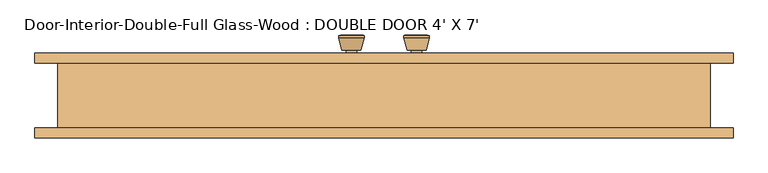
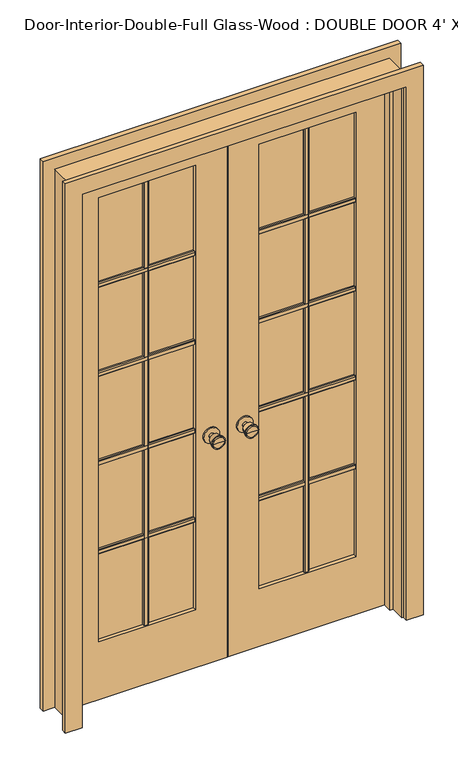
"""IFC4 building model written with IfcOpenShell, lengths in millimetres: door geometry, Door-Interior-Double-Full Glass-Wood : DOUBLE DOOR 4' X 7'."""

from ifc_helpers import new_model, si_unit, point, frame, frame_2d, origin, place, context, project, spatial, polyline, circle_curve, trimmed, segment, composite_curve, outline, extrude, faceted_brep, source, transform, mapped, element, save
from ifc_brep_helpers import plane_surface, cylinder_surface, revolved_surface, advanced_brep


def door_interior_double_full_glass_wood_double_door_4_x_7_060eee9d(model_context):
    return source(origin(), model_context, "Body", "SolidModel", [
        advanced_brep(
        [(-63.5, 66.325, 914.4), (-73.5, 66.325, 914.4), (-53.5, 66.325, 914.4), (-83.9758676, 115.325, 914.4), (-63.5, 115.325, 914.4), (-43.0241324, 115.325, 914.4), (-88.5, 113.4971319, 914.4), (-38.5, 113.4971319, 914.4), (-88.5, 110.0334537, 914.4), (-38.5, 110.0334537, 914.4), (-82.136236, 85.325, 914.4), (-44.863764, 85.325, 914.4), (-73.5, 85.325, 914.4), (-53.5, 85.325, 914.4)],
        [
            (0, 1),
            (1, 2, circle_curve(frame((-63.5, 66.325, 914.4), z_axis=(0.0, -1.0, 0.0), x_axis=(1.0, 0.0, 0.0)), 10.0)),
            (2, 0),
            (2, 1, circle_curve(frame((-63.5, 66.325, 914.4), z_axis=(0.0, -1.0, 0.0), x_axis=(1.0, 0.0, 0.0)), 10.0)),
            (3, 4),
            (4, 5),
            (5, 3, circle_curve(frame((-63.5, 115.325, 914.4), z_axis=(0.0, 1.0, 0.0), x_axis=(1.0, 0.0, 0.0)), 20.4758676)),
            (3, 5, circle_curve(frame((-63.5, 115.325, 914.4), z_axis=(0.0, 1.0, 0.0), x_axis=(1.0, 0.0, 0.0)), 20.4758676)),
            (6, 3),
            (5, 7),
            (7, 6, circle_curve(frame((-63.5, 113.4971319, 914.4), z_axis=(0.0, 1.0, 0.0), x_axis=(1.0, 0.0, 0.0)), 25.0)),
            (6, 7, circle_curve(frame((-63.5, 113.4971319, 914.4), z_axis=(0.0, 1.0, 0.0), x_axis=(1.0, 0.0, 0.0)), 25.0)),
            (8, 6),
            (7, 9),
            (9, 8, circle_curve(frame((-63.5, 110.0334537, 914.4), z_axis=(0.0, 1.0, 0.0), x_axis=(1.0, 0.0, 0.0)), 25.0)),
            (8, 9, circle_curve(frame((-63.5, 110.0334537, 914.4), z_axis=(0.0, 1.0, 0.0), x_axis=(1.0, 0.0, 0.0)), 25.0)),
            (10, 8),
            (9, 11),
            (11, 10, circle_curve(frame((-63.5, 85.325, 914.4), z_axis=(0.0, 1.0, 0.0), x_axis=(1.0, 0.0, 0.0)), 18.636236)),
            (10, 11, circle_curve(frame((-63.5, 85.325, 914.4), z_axis=(0.0, 1.0, 0.0), x_axis=(1.0, 0.0, 0.0)), 18.636236)),
            (12, 10),
            (11, 13),
            (13, 12, circle_curve(frame((-63.5, 85.325, 914.4), z_axis=(0.0, 1.0, 0.0), x_axis=(1.0, 0.0, 0.0)), 10.0)),
            (12, 13, circle_curve(frame((-63.5, 85.325, 914.4), z_axis=(0.0, 1.0, 0.0), x_axis=(1.0, 0.0, 0.0)), 10.0)),
            (1, 12),
            (13, 2),
        ],
        [
            plane_surface(frame((-63.5, 66.325, 914.4), z_axis=(0.0, -1.0, 0.0), x_axis=(1.0, 0.0, 0.0))),
            plane_surface(frame((-63.5, 115.325, 914.4), z_axis=(0.0, 1.0, 0.0), x_axis=(1.0, 0.0, 0.0))),
            revolved_surface(polyline([(-43.0241324, 115.325, 914.4), (-38.5, 113.4971319, 914.4)]), (-63.5, 66.325, 914.4), (0.0, -1.0, 0.0)),
            cylinder_surface(frame((-63.5, 66.325, 914.4), z_axis=(0.0, -1.0, 0.0), x_axis=(1.0, 0.0, 0.0)), 25.0),
            revolved_surface(polyline([(-38.5, 110.0334537, 914.4), (-44.863764, 85.325, 914.4)]), (-63.5, 66.325, 914.4), (0.0, -1.0, 0.0)),
            plane_surface(frame((-63.5, 85.325, 914.4), z_axis=(0.0, -1.0, 0.0), x_axis=(1.0, 0.0, 0.0))),
            cylinder_surface(frame((-63.5, 66.325, 914.4), z_axis=(0.0, -1.0, 0.0), x_axis=(1.0, 0.0, 0.0)), 10.0),
        ],
        [
            (0, [[1, 2, 3]]),
            (0, [[-3, 4, -1]]),
            (1, [[5, 6, 7]]),
            (1, [[-6, -5, 8]]),
            (2, [[9, -7, 10, 11]]),
            (2, [[-10, -8, -9, 12]]),
            (3, [[13, -11, 14, 15]]),
            (3, [[-14, -12, -13, 16]]),
            (4, [[17, -15, 18, 19]]),
            (4, [[-18, -16, -17, 20]]),
            (5, [[21, -19, 22, 23]]),
            (5, [[-22, -20, -21, 24]]),
            (6, [[25, -23, 26, -2]]),
            (6, [[-26, -24, -25, -4]]),
        ],
    ),
        extrude(outline(composite_curve([segment(trimmed(circle_curve(frame_2d((914.4, -63.5)), 30.0), [point((914.4, -33.5))], [point((914.4, -93.5))], False, "CARTESIAN"), True, "CONTINUOUS"), segment(trimmed(circle_curve(frame_2d((914.4, -63.5)), 30.0), [point((914.4, -93.5))], [point((914.4, -33.5))], False, "CARTESIAN"), True, "CONTINUOUS")], self_intersect=False)), frame((0.0, 60.325, 0.0), z_axis=(0.0, 1.0, 0.0), x_axis=(0.0, 0.0, 1.0)), (0.0, 0.0, 1.0), 6.0),
        advanced_brep(
        [(-63.5, 19.4, 914.4), (-53.5, 19.4, 914.4), (-73.5, 19.4, 914.4), (-83.9758676, -29.6, 914.4), (-43.0241324, -29.6, 914.4), (-63.5, -29.6, 914.4), (-88.5, -27.7721319, 914.4), (-38.5, -27.7721319, 914.4), (-88.5, -24.3084537, 914.4), (-38.5, -24.3084537, 914.4), (-82.136236, 0.4, 914.4), (-44.863764, 0.4, 914.4), (-73.5, 0.4, 914.4), (-53.5, 0.4, 914.4)],
        [
            (0, 1),
            (1, 2, circle_curve(frame((-63.5, 19.4, 914.4), z_axis=(0.0, 1.0, 0.0), x_axis=(1.0, 0.0, 0.0)), 10.0)),
            (2, 0),
            (2, 1, circle_curve(frame((-63.5, 19.4, 914.4), z_axis=(0.0, 1.0, 0.0), x_axis=(1.0, 0.0, 0.0)), 10.0)),
            (3, 4, circle_curve(frame((-63.5, -29.6, 914.4), z_axis=(0.0, -1.0, 0.0), x_axis=(1.0, 0.0, 0.0)), 20.4758676)),
            (4, 5),
            (5, 3),
            (4, 3, circle_curve(frame((-63.5, -29.6, 914.4), z_axis=(0.0, -1.0, 0.0), x_axis=(1.0, 0.0, 0.0)), 20.4758676)),
            (6, 7, circle_curve(frame((-63.5, -27.7721319, 914.4), z_axis=(0.0, -1.0, 0.0), x_axis=(1.0, 0.0, 0.0)), 25.0)),
            (7, 4),
            (3, 6),
            (7, 6, circle_curve(frame((-63.5, -27.7721319, 914.4), z_axis=(0.0, -1.0, 0.0), x_axis=(1.0, 0.0, 0.0)), 25.0)),
            (8, 9, circle_curve(frame((-63.5, -24.3084537, 914.4), z_axis=(0.0, -1.0, 0.0), x_axis=(1.0, 0.0, 0.0)), 25.0)),
            (9, 7),
            (6, 8),
            (9, 8, circle_curve(frame((-63.5, -24.3084537, 914.4), z_axis=(0.0, -1.0, 0.0), x_axis=(1.0, 0.0, 0.0)), 25.0)),
            (10, 11, circle_curve(frame((-63.5, 0.4, 914.4), z_axis=(0.0, -1.0, 0.0), x_axis=(1.0, 0.0, 0.0)), 18.636236)),
            (11, 9),
            (8, 10),
            (11, 10, circle_curve(frame((-63.5, 0.4, 914.4), z_axis=(0.0, -1.0, 0.0), x_axis=(1.0, 0.0, 0.0)), 18.636236)),
            (12, 13, circle_curve(frame((-63.5, 0.4, 914.4), z_axis=(0.0, -1.0, 0.0), x_axis=(1.0, 0.0, 0.0)), 10.0)),
            (13, 11),
            (10, 12),
            (13, 12, circle_curve(frame((-63.5, 0.4, 914.4), z_axis=(0.0, -1.0, 0.0), x_axis=(1.0, 0.0, 0.0)), 10.0)),
            (1, 13),
            (12, 2),
        ],
        [
            plane_surface(frame((-63.5, 19.4, 914.4), z_axis=(0.0, 1.0, 0.0), x_axis=(1.0, 0.0, 0.0))),
            plane_surface(frame((-63.5, -29.6, 914.4), z_axis=(0.0, -1.0, 0.0), x_axis=(1.0, 0.0, 0.0))),
            revolved_surface(polyline([(-43.0241324, -29.6, 914.4), (-38.5, -27.7721319, 914.4)]), (-63.5, 19.4, 914.4), (0.0, 1.0, 0.0)),
            cylinder_surface(frame((-63.5, 19.4, 914.4), z_axis=(0.0, 1.0, 0.0), x_axis=(1.0, 0.0, 0.0)), 25.0),
            revolved_surface(polyline([(-38.5, -24.3084537, 914.4), (-44.863764, 0.4, 914.4)]), (-63.5, 19.4, 914.4), (0.0, 1.0, 0.0)),
            plane_surface(frame((-63.5, 0.4, 914.4), z_axis=(0.0, 1.0, 0.0), x_axis=(1.0, 0.0, 0.0))),
            cylinder_surface(frame((-63.5, 19.4, 914.4), z_axis=(0.0, 1.0, 0.0), x_axis=(1.0, 0.0, 0.0)), 10.0),
        ],
        [
            (0, [[1, 2, 3]]),
            (0, [[-3, 4, -1]]),
            (1, [[5, 6, 7]]),
            (1, [[8, -7, -6]]),
            (2, [[9, 10, -5, 11]]),
            (2, [[12, -11, -8, -10]]),
            (3, [[13, 14, -9, 15]]),
            (3, [[16, -15, -12, -14]]),
            (4, [[17, 18, -13, 19]]),
            (4, [[20, -19, -16, -18]]),
            (5, [[21, 22, -17, 23]]),
            (5, [[24, -23, -20, -22]]),
            (6, [[-2, 25, -21, 26]]),
            (6, [[-4, -26, -24, -25]]),
        ],
    ),
        extrude(outline(composite_curve([segment(trimmed(circle_curve(frame_2d((914.4, -63.5)), 30.0), [point((914.4, -33.5))], [point((914.4, -93.5))], False, "CARTESIAN"), True, "CONTINUOUS"), segment(trimmed(circle_curve(frame_2d((914.4, -63.5)), 30.0), [point((914.4, -93.5))], [point((914.4, -33.5))], False, "CARTESIAN"), True, "CONTINUOUS")], self_intersect=False)), frame((0.0, 19.4, 0.0), z_axis=(0.0, 1.0, 0.0), x_axis=(0.0, 0.0, 1.0)), (0.0, 0.0, 1.0), 6.0),
        extrude(outline(polyline([(39.37, 1667.51), (39.37, 1648.46), (33.02, 1648.46), (29.845, 1651.635), (29.845, 1664.335), (33.02, 1667.51), (39.37, 1667.51)])), frame((120.65, 0.0, 0.0), z_axis=(1.0, 0.0, 0.0), x_axis=(0.0, 1.0, 0.0)), (0.0, 0.0, 1.0), 368.3),
        extrude(outline(polyline([(39.37, 1310.9575), (39.37, 1291.9075), (33.02, 1291.9075), (29.845, 1295.0825), (29.845, 1307.7825), (33.02, 1310.9575), (39.37, 1310.9575)])), frame((120.65, 0.0, 0.0), z_axis=(1.0, 0.0, 0.0), x_axis=(0.0, 1.0, 0.0)), (0.0, 0.0, 1.0), 368.3),
        extrude(outline(polyline([(39.37, 954.405), (39.37, 935.355), (33.02, 935.355), (29.845, 938.53), (29.845, 951.23), (33.02, 954.405), (39.37, 954.405)])), frame((120.65, 0.0, 0.0), z_axis=(1.0, 0.0, 0.0), x_axis=(0.0, 1.0, 0.0)), (0.0, 0.0, 1.0), 368.3),
        extrude(outline(polyline([(295.275, 39.37), (314.325, 39.37), (314.325, 33.02), (311.15, 29.845), (298.45, 29.845), (295.275, 33.02), (295.275, 39.37)])), frame((0.0, 0.0, 231.775), z_axis=(0.0, 0.0, 1.0), x_axis=(1.0, 0.0, 0.0)), (0.0, 0.0, 1.0), 1782.7625),
        extrude(outline(polyline([(39.37, 597.8525), (39.37, 578.8025), (33.02, 578.8025), (29.845, 581.9775), (29.845, 594.6775), (33.02, 597.8525), (39.37, 597.8525)])), frame((120.65, 0.0, 0.0), z_axis=(1.0, 0.0, 0.0), x_axis=(0.0, 1.0, 0.0)), (0.0, 0.0, 1.0), 368.3),
        extrude(outline(polyline([(46.355, 1667.51), (52.705, 1667.51), (55.88, 1664.335), (55.88, 1651.635), (52.705, 1648.46), (46.355, 1648.46), (46.355, 1667.51)])), frame((-488.95, 0.0, 0.0), z_axis=(1.0, 0.0, 0.0), x_axis=(0.0, 1.0, 0.0)), (0.0, 0.0, 1.0), 368.3),
        extrude(outline(polyline([(46.355, 1310.9575), (52.705, 1310.9575), (55.88, 1307.7825), (55.88, 1295.0825), (52.705, 1291.9075), (46.355, 1291.9075), (46.355, 1310.9575)])), frame((-488.95, 0.0, 0.0), z_axis=(1.0, 0.0, 0.0), x_axis=(0.0, 1.0, 0.0)), (0.0, 0.0, 1.0), 368.3),
        extrude(outline(polyline([(46.355, 954.405), (52.705, 954.405), (55.88, 951.23), (55.88, 938.53), (52.705, 935.355), (46.355, 935.355), (46.355, 954.405)])), frame((-488.95, 0.0, 0.0), z_axis=(1.0, 0.0, 0.0), x_axis=(0.0, 1.0, 0.0)), (0.0, 0.0, 1.0), 368.3),
        extrude(outline(polyline([(-314.325, 46.355), (-314.325, 52.705), (-311.15, 55.88), (-298.45, 55.88), (-295.275, 52.705), (-295.275, 46.355), (-314.325, 46.355)])), frame((0.0, 0.0, 231.775), z_axis=(0.0, 0.0, 1.0), x_axis=(1.0, 0.0, 0.0)), (0.0, 0.0, 1.0), 1782.7625),
        extrude(outline(polyline([(46.355, 597.8525), (52.705, 597.8525), (55.88, 594.6775), (55.88, 581.9775), (52.705, 578.8025), (46.355, 578.8025), (46.355, 597.8525)])), frame((-488.95, 0.0, 0.0), z_axis=(1.0, 0.0, 0.0), x_axis=(0.0, 1.0, 0.0)), (0.0, 0.0, 1.0), 368.3),
        extrude(outline(polyline([(46.355, 1667.51), (52.705, 1667.51), (55.88, 1664.335), (55.88, 1651.635), (52.705, 1648.46), (46.355, 1648.46), (46.355, 1667.51)])), frame((120.65, 0.0, 0.0), z_axis=(1.0, 0.0, 0.0), x_axis=(0.0, 1.0, 0.0)), (0.0, 0.0, 1.0), 368.3),
        extrude(outline(polyline([(46.355, 1310.9575), (52.705, 1310.9575), (55.88, 1307.7825), (55.88, 1295.0825), (52.705, 1291.9075), (46.355, 1291.9075), (46.355, 1310.9575)])), frame((120.65, 0.0, 0.0), z_axis=(1.0, 0.0, 0.0), x_axis=(0.0, 1.0, 0.0)), (0.0, 0.0, 1.0), 368.3),
        extrude(outline(polyline([(46.355, 954.405), (52.705, 954.405), (55.88, 951.23), (55.88, 938.53), (52.705, 935.355), (46.355, 935.355), (46.355, 954.405)])), frame((120.65, 0.0, 0.0), z_axis=(1.0, 0.0, 0.0), x_axis=(0.0, 1.0, 0.0)), (0.0, 0.0, 1.0), 368.3),
        extrude(outline(polyline([(295.275, 46.355), (295.275, 52.705), (298.45, 55.88), (311.15, 55.88), (314.325, 52.705), (314.325, 46.355), (295.275, 46.355)])), frame((0.0, 0.0, 231.775), z_axis=(0.0, 0.0, 1.0), x_axis=(1.0, 0.0, 0.0)), (0.0, 0.0, 1.0), 1782.7625),
        extrude(outline(polyline([(46.355, 597.8525), (52.705, 597.8525), (55.88, 594.6775), (55.88, 581.9775), (52.705, 578.8025), (46.355, 578.8025), (46.355, 597.8525)])), frame((120.65, 0.0, 0.0), z_axis=(1.0, 0.0, 0.0), x_axis=(0.0, 1.0, 0.0)), (0.0, 0.0, 1.0), 368.3),
        extrude(outline(polyline([(39.37, 1667.51), (39.37, 1648.46), (33.02, 1648.46), (29.845, 1651.635), (29.845, 1664.335), (33.02, 1667.51), (39.37, 1667.51)])), frame((-488.95, 0.0, 0.0), z_axis=(1.0, 0.0, 0.0), x_axis=(0.0, 1.0, 0.0)), (0.0, 0.0, 1.0), 368.3),
        extrude(outline(polyline([(39.37, 1310.9575), (39.37, 1291.9075), (33.02, 1291.9075), (29.845, 1295.0825), (29.845, 1307.7825), (33.02, 1310.9575), (39.37, 1310.9575)])), frame((-488.95, 0.0, 0.0), z_axis=(1.0, 0.0, 0.0), x_axis=(0.0, 1.0, 0.0)), (0.0, 0.0, 1.0), 368.3),
        extrude(outline(polyline([(39.37, 954.405), (39.37, 935.355), (33.02, 935.355), (29.845, 938.53), (29.845, 951.23), (33.02, 954.405), (39.37, 954.405)])), frame((-488.95, 0.0, 0.0), z_axis=(1.0, 0.0, 0.0), x_axis=(0.0, 1.0, 0.0)), (0.0, 0.0, 1.0), 368.3),
        extrude(outline(polyline([(-314.325, 39.37), (-295.275, 39.37), (-295.275, 33.02), (-298.45, 29.845), (-311.15, 29.845), (-314.325, 33.02), (-314.325, 39.37)])), frame((0.0, 0.0, 231.775), z_axis=(0.0, 0.0, 1.0), x_axis=(1.0, 0.0, 0.0)), (0.0, 0.0, 1.0), 1782.7625),
        extrude(outline(polyline([(39.37, 597.8525), (39.37, 578.8025), (33.02, 578.8025), (29.845, 581.9775), (29.845, 594.6775), (33.02, 597.8525), (39.37, 597.8525)])), frame((-488.95, 0.0, 0.0), z_axis=(1.0, 0.0, 0.0), x_axis=(0.0, 1.0, 0.0)), (0.0, 0.0, 1.0), 368.3),
        advanced_brep(
        [(63.5, 19.4, 914.4), (73.5, 19.4, 914.4), (53.5, 19.4, 914.4), (83.9758676, -29.6, 914.4), (63.5, -29.6, 914.4), (43.0241324, -29.6, 914.4), (88.5, -27.7721319, 914.4), (38.5, -27.7721319, 914.4), (88.5, -24.3084537, 914.4), (38.5, -24.3084537, 914.4), (82.136236, 0.4, 914.4), (44.863764, 0.4, 914.4), (73.5, 0.4, 914.4), (53.5, 0.4, 914.4)],
        [
            (0, 1),
            (1, 2, circle_curve(frame((63.5, 19.4, 914.4), z_axis=(0.0, 1.0, 0.0), x_axis=(-1.0, 0.0, 0.0)), 10.0)),
            (2, 0),
            (2, 1, circle_curve(frame((63.5, 19.4, 914.4), z_axis=(0.0, 1.0, 0.0), x_axis=(-1.0, 0.0, 0.0)), 10.0)),
            (3, 4),
            (4, 5),
            (5, 3, circle_curve(frame((63.5, -29.6, 914.4), z_axis=(0.0, -1.0, 0.0), x_axis=(-1.0, 0.0, 0.0)), 20.4758676)),
            (3, 5, circle_curve(frame((63.5, -29.6, 914.4), z_axis=(0.0, -1.0, 0.0), x_axis=(-1.0, 0.0, 0.0)), 20.4758676)),
            (6, 3),
            (5, 7),
            (7, 6, circle_curve(frame((63.5, -27.7721319, 914.4), z_axis=(0.0, -1.0, 0.0), x_axis=(-1.0, 0.0, 0.0)), 25.0)),
            (6, 7, circle_curve(frame((63.5, -27.7721319, 914.4), z_axis=(0.0, -1.0, 0.0), x_axis=(-1.0, 0.0, 0.0)), 25.0)),
            (8, 6),
            (7, 9),
            (9, 8, circle_curve(frame((63.5, -24.3084537, 914.4), z_axis=(0.0, -1.0, 0.0), x_axis=(-1.0, 0.0, 0.0)), 25.0)),
            (8, 9, circle_curve(frame((63.5, -24.3084537, 914.4), z_axis=(0.0, -1.0, 0.0), x_axis=(-1.0, 0.0, 0.0)), 25.0)),
            (10, 8),
            (9, 11),
            (11, 10, circle_curve(frame((63.5, 0.4, 914.4), z_axis=(0.0, -1.0, 0.0), x_axis=(-1.0, 0.0, 0.0)), 18.636236)),
            (10, 11, circle_curve(frame((63.5, 0.4, 914.4), z_axis=(0.0, -1.0, 0.0), x_axis=(-1.0, 0.0, 0.0)), 18.636236)),
            (12, 10),
            (11, 13),
            (13, 12, circle_curve(frame((63.5, 0.4, 914.4), z_axis=(0.0, -1.0, 0.0), x_axis=(-1.0, 0.0, 0.0)), 10.0)),
            (12, 13, circle_curve(frame((63.5, 0.4, 914.4), z_axis=(0.0, -1.0, 0.0), x_axis=(-1.0, 0.0, 0.0)), 10.0)),
            (1, 12),
            (13, 2),
        ],
        [
            plane_surface(frame((63.5, 19.4, 914.4), z_axis=(0.0, 1.0, 0.0), x_axis=(-1.0, 0.0, 0.0))),
            plane_surface(frame((63.5, -29.6, 914.4), z_axis=(0.0, -1.0, 0.0), x_axis=(-1.0, 0.0, 0.0))),
            revolved_surface(polyline([(43.0241324, -29.6, 914.4), (38.5, -27.7721319, 914.4)]), (63.5, 19.4, 914.4), (0.0, 1.0, 0.0)),
            cylinder_surface(frame((63.5, 19.4, 914.4), z_axis=(0.0, 1.0, 0.0), x_axis=(-1.0, 0.0, 0.0)), 25.0),
            revolved_surface(polyline([(38.5, -24.3084537, 914.4), (44.863764, 0.4, 914.4)]), (63.5, 19.4, 914.4), (0.0, 1.0, 0.0)),
            plane_surface(frame((63.5, 0.4, 914.4), z_axis=(0.0, 1.0, 0.0), x_axis=(-1.0, 0.0, 0.0))),
            cylinder_surface(frame((63.5, 19.4, 914.4), z_axis=(0.0, 1.0, 0.0), x_axis=(-1.0, 0.0, 0.0)), 10.0),
        ],
        [
            (0, [[1, 2, 3]]),
            (0, [[-3, 4, -1]]),
            (1, [[5, 6, 7]]),
            (1, [[-6, -5, 8]]),
            (2, [[9, -7, 10, 11]]),
            (2, [[-10, -8, -9, 12]]),
            (3, [[13, -11, 14, 15]]),
            (3, [[-14, -12, -13, 16]]),
            (4, [[17, -15, 18, 19]]),
            (4, [[-18, -16, -17, 20]]),
            (5, [[21, -19, 22, 23]]),
            (5, [[-22, -20, -21, 24]]),
            (6, [[25, -23, 26, -2]]),
            (6, [[-26, -24, -25, -4]]),
        ],
    ),
        extrude(outline(composite_curve([segment(trimmed(circle_curve(frame_2d((914.4, 63.5)), 30.0), [point((914.4, 33.5))], [point((914.4, 93.5))], False, "CARTESIAN"), True, "CONTINUOUS"), segment(trimmed(circle_curve(frame_2d((914.4, 63.5)), 30.0), [point((914.4, 93.5))], [point((914.4, 33.5))], False, "CARTESIAN"), True, "CONTINUOUS")], self_intersect=False)), frame((0.0, 19.4, 0.0), z_axis=(0.0, 1.0, 0.0), x_axis=(0.0, 0.0, 1.0)), (0.0, 0.0, 1.0), 6.0),
        advanced_brep(
        [(63.5, 66.325, 914.4), (53.5, 66.325, 914.4), (73.5, 66.325, 914.4), (83.9758676, 115.325, 914.4), (43.0241324, 115.325, 914.4), (63.5, 115.325, 914.4), (88.5, 113.4971319, 914.4), (38.5, 113.4971319, 914.4), (88.5, 110.0334537, 914.4), (38.5, 110.0334537, 914.4), (82.136236, 85.325, 914.4), (44.863764, 85.325, 914.4), (73.5, 85.325, 914.4), (53.5, 85.325, 914.4)],
        [
            (0, 1),
            (1, 2, circle_curve(frame((63.5, 66.325, 914.4), z_axis=(0.0, -1.0, 0.0), x_axis=(-1.0, 0.0, 0.0)), 10.0)),
            (2, 0),
            (2, 1, circle_curve(frame((63.5, 66.325, 914.4), z_axis=(0.0, -1.0, 0.0), x_axis=(-1.0, 0.0, 0.0)), 10.0)),
            (3, 4, circle_curve(frame((63.5, 115.325, 914.4), z_axis=(0.0, 1.0, 0.0), x_axis=(-1.0, 0.0, 0.0)), 20.4758676)),
            (4, 5),
            (5, 3),
            (4, 3, circle_curve(frame((63.5, 115.325, 914.4), z_axis=(0.0, 1.0, 0.0), x_axis=(-1.0, 0.0, 0.0)), 20.4758676)),
            (6, 7, circle_curve(frame((63.5, 113.4971319, 914.4), z_axis=(0.0, 1.0, 0.0), x_axis=(-1.0, 0.0, 0.0)), 25.0)),
            (7, 4),
            (3, 6),
            (7, 6, circle_curve(frame((63.5, 113.4971319, 914.4), z_axis=(0.0, 1.0, 0.0), x_axis=(-1.0, 0.0, 0.0)), 25.0)),
            (8, 9, circle_curve(frame((63.5, 110.0334537, 914.4), z_axis=(0.0, 1.0, 0.0), x_axis=(-1.0, 0.0, 0.0)), 25.0)),
            (9, 7),
            (6, 8),
            (9, 8, circle_curve(frame((63.5, 110.0334537, 914.4), z_axis=(0.0, 1.0, 0.0), x_axis=(-1.0, 0.0, 0.0)), 25.0)),
            (10, 11, circle_curve(frame((63.5, 85.325, 914.4), z_axis=(0.0, 1.0, 0.0), x_axis=(-1.0, 0.0, 0.0)), 18.636236)),
            (11, 9),
            (8, 10),
            (11, 10, circle_curve(frame((63.5, 85.325, 914.4), z_axis=(0.0, 1.0, 0.0), x_axis=(-1.0, 0.0, 0.0)), 18.636236)),
            (12, 13, circle_curve(frame((63.5, 85.325, 914.4), z_axis=(0.0, 1.0, 0.0), x_axis=(-1.0, 0.0, 0.0)), 10.0)),
            (13, 11),
            (10, 12),
            (13, 12, circle_curve(frame((63.5, 85.325, 914.4), z_axis=(0.0, 1.0, 0.0), x_axis=(-1.0, 0.0, 0.0)), 10.0)),
            (1, 13),
            (12, 2),
        ],
        [
            plane_surface(frame((63.5, 66.325, 914.4), z_axis=(0.0, -1.0, 0.0), x_axis=(-1.0, 0.0, 0.0))),
            plane_surface(frame((63.5, 115.325, 914.4), z_axis=(0.0, 1.0, 0.0), x_axis=(-1.0, 0.0, 0.0))),
            revolved_surface(polyline([(43.0241324, 115.325, 914.4), (38.5, 113.4971319, 914.4)]), (63.5, 66.325, 914.4), (0.0, -1.0, 0.0)),
            cylinder_surface(frame((63.5, 66.325, 914.4), z_axis=(0.0, -1.0, 0.0), x_axis=(-1.0, 0.0, 0.0)), 25.0),
            revolved_surface(polyline([(38.5, 110.0334537, 914.4), (44.863764, 85.325, 914.4)]), (63.5, 66.325, 914.4), (0.0, -1.0, 0.0)),
            plane_surface(frame((63.5, 85.325, 914.4), z_axis=(0.0, -1.0, 0.0), x_axis=(-1.0, 0.0, 0.0))),
            cylinder_surface(frame((63.5, 66.325, 914.4), z_axis=(0.0, -1.0, 0.0), x_axis=(-1.0, 0.0, 0.0)), 10.0),
        ],
        [
            (0, [[1, 2, 3]]),
            (0, [[-3, 4, -1]]),
            (1, [[5, 6, 7]]),
            (1, [[8, -7, -6]]),
            (2, [[9, 10, -5, 11]]),
            (2, [[12, -11, -8, -10]]),
            (3, [[13, 14, -9, 15]]),
            (3, [[16, -15, -12, -14]]),
            (4, [[17, 18, -13, 19]]),
            (4, [[20, -19, -16, -18]]),
            (5, [[21, 22, -17, 23]]),
            (5, [[24, -23, -20, -22]]),
            (6, [[-2, 25, -21, 26]]),
            (6, [[-4, -26, -24, -25]]),
        ],
    ),
        extrude(outline(composite_curve([segment(trimmed(circle_curve(frame_2d((914.4, 63.5)), 30.0), [point((914.4, 33.5))], [point((914.4, 93.5))], False, "CARTESIAN"), True, "CONTINUOUS"), segment(trimmed(circle_curve(frame_2d((914.4, 63.5)), 30.0), [point((914.4, 93.5))], [point((914.4, 33.5))], False, "CARTESIAN"), True, "CONTINUOUS")], self_intersect=False)), frame((0.0, 60.325, 0.0), z_axis=(0.0, 1.0, 0.0), x_axis=(0.0, 0.0, 1.0)), (0.0, 0.0, 1.0), 6.0),
        extrude(outline(polyline([(0.0, 615.95), (0.0, 679.45), (2203.45, 679.45), (2203.45, -679.45), (0.0, -679.45), (0.0, -615.95), (2139.95, -615.95), (2139.95, 615.95), (0.0, 615.95)])), frame((0.0, -85.725, 0.0), z_axis=(0.0, 1.0, 0.0), x_axis=(0.0, 0.0, 1.0)), (0.0, 0.0, 1.0), 19.05),
        extrude(outline(polyline([(0.0, 615.95), (0.0, 679.45), (2203.45, 679.45), (2203.45, -679.45), (0.0, -679.45), (0.0, -615.95), (2139.95, -615.95), (2139.95, 615.95), (0.0, 615.95)])), frame((0.0, 60.325, 0.0), z_axis=(0.0, 1.0, 0.0), x_axis=(0.0, 0.0, 1.0)), (0.0, 0.0, 1.0), 19.05),
        faceted_brep([(635.0, 60.325, 0.0), (635.0, -66.675, 0.0), (609.6, -66.675, 0.0), (609.6, -9.525, 0.0), (596.9, -9.525, 0.0), (596.9, 25.4, 0.0), (609.6, 25.4, 0.0), (609.6, 60.325, 0.0), (635.0, 60.325, 2159.0), (635.0, -66.675, 2159.0), (-635.0, -66.675, 2159.0), (-635.0, -66.675, 0.0), (-609.6, -66.675, 0.0), (-609.6, -66.675, 2133.6), (609.6, -66.675, 2133.6), (609.6, -9.525, 2133.6), (-609.6, -9.525, 2133.6), (-609.6, -9.525, 0.0), (-596.9, -9.525, 0.0), (-596.9, -9.525, 2120.9), (596.9, -9.525, 2120.9), (596.9, 25.4, 2120.9), (1.5875, 25.4, 2120.9), (-1.6019111, 25.4, 2120.9), (-596.9, 25.4, 2120.9), (-596.9, 25.4, 0.0), (-609.6, 25.4, 0.0), (-609.6, 25.4, 2133.6), (-1.6019111, 25.4, 2133.6), (1.5875, 25.4, 2133.6), (609.6, 25.4, 2133.6), (609.6, 60.325, 2133.6), (1.5875, 60.325, 2133.6), (-1.6019111, 60.325, 2133.6), (-609.6, 60.325, 2133.6), (-609.6, 60.325, 0.0), (-635.0, 60.325, 0.0), (-635.0, 60.325, 2159.0)], [[[0, 1, 2, 3, 4, 5, 6, 7]], [[1, 0, 8, 9]], [[2, 1, 9, 10, 11, 12, 13, 14]], [[3, 2, 14, 15]], [[4, 3, 15, 16, 17, 18, 19, 20]], [[5, 4, 20, 21]], [[6, 5, 21, 22, 23, 24, 25, 26, 27, 28, 29, 30]], [[7, 6, 30, 31]], [[0, 7, 31, 32, 33, 34, 35, 36, 37, 8]], [[9, 8, 37, 10]], [[14, 13, 16, 15]], [[20, 19, 24, 23, 22, 21]], [[31, 30, 29, 28, 27, 34, 33, 32]], [[12, 11, 36, 35, 26, 25, 18, 17]], [[11, 10, 37, 36]], [[13, 12, 17, 16]], [[19, 18, 25, 24]], [[27, 26, 35, 34]]]),
        extrude(outline(polyline([(2133.6, -609.6), (0.0, -609.6), (0.0, -1.6019111), (2133.6, -1.6019111), (2133.6, -609.6)]), holes=[polyline([(231.775, -488.95), (2014.5375, -488.95), (2014.5375, -120.65), (231.775, -120.65), (231.775, -488.95)])]), frame((0.0, 25.4, 0.0), z_axis=(0.0, 1.0, 0.0), x_axis=(0.0, 0.0, 1.0)), (0.0, 0.0, 1.0), 34.925),
        extrude(outline(polyline([(0.0, 609.6), (2133.6, 609.6), (2133.6, 1.5875), (0.0, 1.5875), (0.0, 609.6)]), holes=[polyline([(2014.5375, 120.65), (2014.5375, 488.95), (231.775, 488.95), (231.775, 120.65), (2014.5375, 120.65)])]), frame((0.0, 25.4, 0.0), z_axis=(0.0, 1.0, 0.0), x_axis=(0.0, 0.0, 1.0)), (0.0, 0.0, 1.0), 34.925),
        extrude(outline(polyline([(488.95, 39.37), (120.65, 39.37), (120.65, 46.355), (488.95, 46.355), (488.95, 39.37)])), frame((0.0, 0.0, 231.775), z_axis=(0.0, 0.0, 1.0), x_axis=(1.0, 0.0, 0.0)), (0.0, 0.0, 1.0), 1782.7625),
        extrude(outline(polyline([(-120.65, 39.37), (-488.95, 39.37), (-488.95, 46.355), (-120.65, 46.355), (-120.65, 39.37)])), frame((0.0, 0.0, 231.775), z_axis=(0.0, 0.0, 1.0), x_axis=(1.0, 0.0, 0.0)), (0.0, 0.0, 1.0), 1782.7625),
    ])


if __name__ == "__main__":
    model = new_model("IFC4")
    model_context = context("Model", 3, world=origin())
    ifc_project = project(units=[si_unit("LENGTHUNIT", "METRE", prefix="MILLI")], contexts=[model_context])
    site = spatial("IfcSite", under=ifc_project)
    building = spatial("IfcBuilding", under=site)
    placement = place(None, origin())
    door_interior_double_full_glass_wood_double_door_4_x_7_shape = door_interior_double_full_glass_wood_double_door_4_x_7_060eee9d(model_context)
    element("IfcDoor", 1, ObjectType="Door-Interior-Double-Full Glass-Wood : DOUBLE DOOR 4' X 7'", at=placement, inside=building, context=model_context, shape_type="MappedRepresentation", body=[
        mapped(door_interior_double_full_glass_wood_double_door_4_x_7_shape, transform((0.0, 0.0, 0.0), x_axis=(1.0, 0.0, 0.0), y_axis=(0.0, 1.0, 0.0), z_axis=(0.0, 0.0, 1.0))),
    ])
    save(model, "model.ifc")

# Revit data of these elements
# Type "Door-Interior-Double-Full Glass-Wood : DOUBLE DOOR 4' X 7'"
#   Type Mark = "9"
#   Assembly Code = "C1020300"
#   Analytic Construction = "French door, wood frame with single glass"
#   Top Rail = 0' - 4 11/16"
#   Thickness = 0' - 1 3/8"
#   Thermal Resistance (R) = 1.0696 (h·ft²·°F)/BTU
#   Swing Angle [instance default] = 90.00°
#   Stiles = 0' - 4 3/4"
#   Rough Width = 4' - 2"
#   Rough Height = 7' - 1"
#   Panel Width = 2' - 0"
#   Height = 7' - 0"
#   Width = 4' - 0"
#   Heat Transfer Coefficient (U) = 0.9350 BTU/(h·ft²·°F)
#   Bottom Rail = 0' - 9 1/8"
#   Show Grill [instance default] = yes
#   Trim Material = Cherry
#   Panel Material = Cherry
#   Frame Material = Cherry
#   Door Handle Material = Aluminum
#   Visual Light Transmittance = 0
#   Solar Heat Gain Coefficient = 0
#   Wall Closure = (empty or 0)
#   Function = (empty or 0)
# Element 1 (IfcDoor, "Door-Interior-Double-Full Glass-Wood : DOUBLE DOOR 4' X 7'")
#   Materials on its faces: "Cherry", "Aluminum", "Glass"
# Materials
#   "Cherry": class "Wood", colour RGB 226 177 128, transparency 0, Description = "Prunus Serotina", Cost = 0
#   "Aluminum": class "Metal", colour RGB 247 247 247, transparency 0, Description = "Aluminum 6061", Cost = 0
#   "Glass": class "Glass", colour RGB 0 128 192, transparency 0.75, Description = "Soda Lime Glass", Cost = 0
